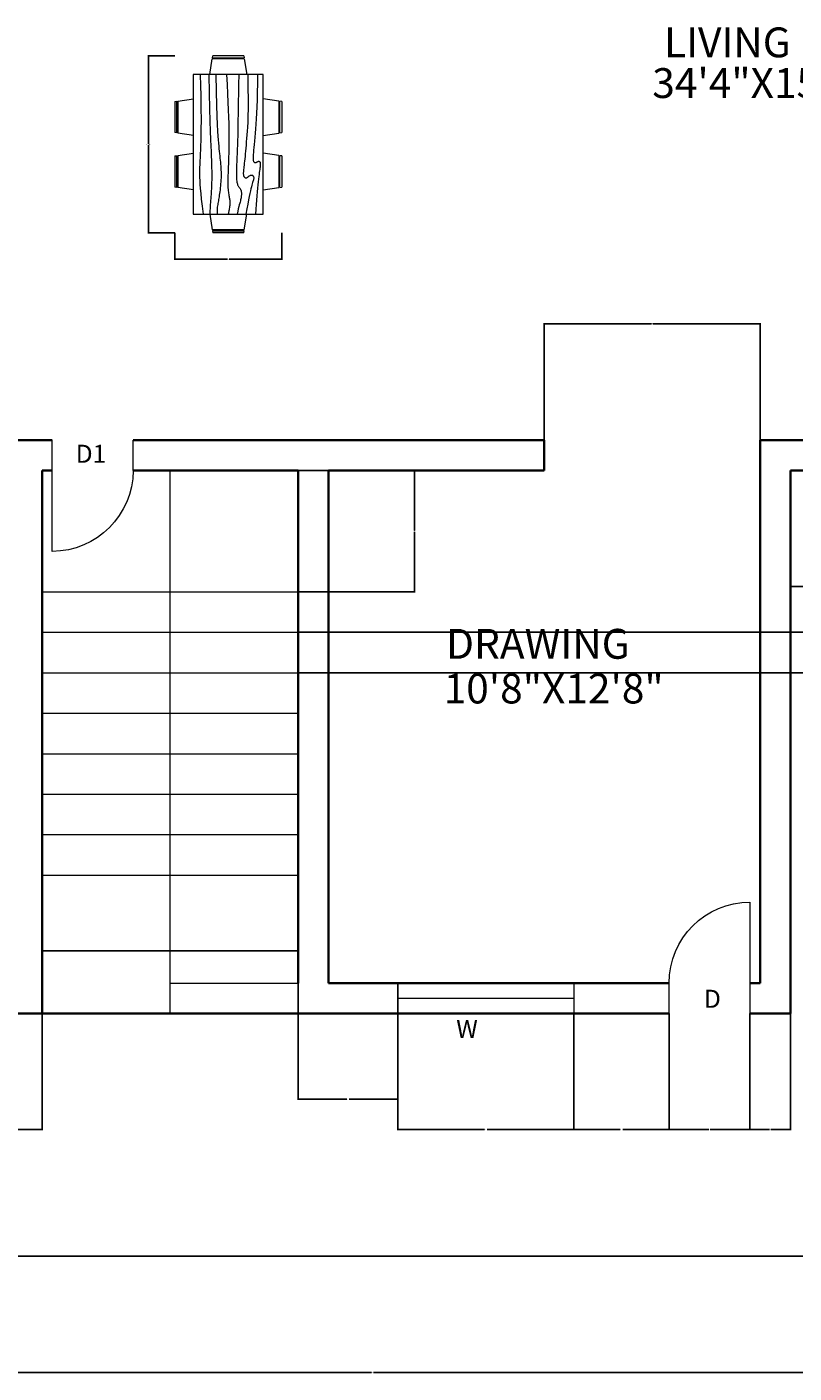
# Model space of a CAD drawing. Units: feet. Extents: x 1508 to 2265, y 1718 to 2421.
# Tile 2 of 4: x 1784 to 2012, y 1718 to 2117. Entities that reach past the tile are written whole.
import ezdxf

# ---------------------------------------------------------------- set-up
doc = ezdxf.new("R2010")
doc.units = ezdxf.units.FT
for name, color, linetype, lineweight in [('A-ANNO-DIMS', 2, 'Continuous', 18), ('A-ANNO-TEXT', 3, 'Continuous', 13), ('A-AREA-IDEN', 7, 'Continuous', 18), ('A-DOOR', 3, 'Continuous', 18), ('A-FLOR-STRS', 2, 'Continuous', 18), ('A-FURN', 8, 'Continuous', 18), ('A-GLAZ', 4, 'Continuous', 18), ('A-WALL', 7, 'Continuous', 35), ('C-PROP', 7, 'Continuous', 25)]:
    doc.layers.add(name, color=color, linetype=linetype, lineweight=lineweight)
doc.styles.get("Standard").update_dxf_attribs({"font": 'arial.ttf'})
doc.dimstyles.get("Standard").update_dxf_attribs({"dimtxt": 0.18, "dimasz": 0.18, "dimexe": 0.18, "dimexo": 0.0625, "dimgap": 0.09, "dimtad": 0, "dimtih": 1, "dimtoh": 1, "dimdec": 4, "dimzin": 0, "dimdsep": 46, "dimtxsty": 'Standard', "dimcen": 0.09, "dimadec": 0, "dimazin": 0, "dimtfac": 1, "dimtdec": 4, "dimtofl": 0, "dimtmove": 0, "dimatfit": 3, "dimfxl": 1, "dimtolj": 1, "dimtzin": 0, "dimarcsym": 0})

# ---------------------------------------------------------------- blocks, each defined once
blk = doc.blocks.new('Dining Set - 36 x 72 in.')
for p, q in [((-22.2343, 26.00059), (-23.4847, 17.99762)), ((-22.2304, 26), (-5.7608, 26)), ((-22, 27.5), (-22.1562, 26.50042)), ((-5.8416, 26.5), (-22.1534, 26.5)), ((-22, 27.5), (-6, 27.5)), ((-5.8437, 26.49966), (-6, 27.5)), ((-4.5152, 17.99762), (-5.7655, 25.99926)), ((5.7657, 26.00059), (4.5153, 17.99762)), ((5.7696, 26), (22.2392, 26)), ((6, 27.5), (5.8438, 26.50042)), ((22.1584, 26.5), (5.8466, 26.5)), ((6, 27.5), (22, 27.5)), ((22.1563, 26.49966), (22, 27.5)), ((23.4848, 17.99762), (22.2345, 25.99926)), ((36, 18), (-36, 18)), ((-36, 18), (-36, -18)), ((36, -18), (36, 18)), ((-45.5, 8), (-44.5004, 8.15617)), ((-45.5, 8), (-45.5, -8)), ((-44.5, -8.15843), (-44.5, 8.15338)), ((-44.0006, 8.23428), (-35.9976, 9.48474)), ((-44, 8.23041), (-44, -8.23915)), ((44.0006, 8.23428), (35.9976, 9.48474)), ((44, 8.23041), (44, -8.23915)), ((44.5, -8.15843), (44.5, 8.15338)), ((45.5, 8), (44.5005, 8.15617)), ((45.5, 8), (45.5, -8)), ((-44.4997, -8.15631), (-45.5, -8)), ((-35.9976, -9.48476), (-43.9993, -8.2345)), ((35.9976, -9.48476), (43.9993, -8.2345)), ((44.4997, -8.15631), (45.5, -8)), ((-36, -18), (36, -18)), ((-22.2343, -26.0006), (-23.4847, -17.99762)), ((-4.5152, -17.99762), (-5.7655, -25.99928)), ((5.7657, -26.0006), (4.5153, -17.99762)), ((23.4848, -17.99762), (22.2345, -25.99928)), ((-22.2304, -26), (-5.7608, -26)), ((-22, -27.5), (-22.1562, -26.50044)), ((-5.8416, -26.5), (-22.1534, -26.5)), ((-22, -27.5), (-6, -27.5)), ((-5.8437, -26.49967), (-6, -27.5)), ((5.7696, -26), (22.2392, -26)), ((6, -27.5), (5.8438, -26.50044)), ((22.1584, -26.5), (5.8466, -26.5)), ((6, -27.5), (22, -27.5)), ((22.1563, -26.49967), (22, -27.5))]:
    blk.add_line(p, q)
for points in [[(-36, 15), (-31.1772, 14.97754), (-26.8079, 14.91406), (-22.8538, 14.81543), (-19.276, 14.6875), (-16.0362, 14.53613), (-13.0957, 14.36718), (-10.4159, 14.18652), (-7.9583, 14), (-5.6904, 13.81315), (-3.6035, 13.63021), (-1.6954, 13.45508), (0.0365, 13.29166), (1.5945, 13.14388), (2.9811, 13.01562), (4.1988, 12.9108), (5.25, 12.83333), (6.1393, 12.78613), (6.8802, 12.76823), (7.4883, 12.77767), (7.9792, 12.8125), (8.3685, 12.87077), (8.6719, 12.95052), (8.9049, 13.0498), (9.0833, 13.16666), (9.2205, 13.29899), (9.3216, 13.44401), (9.3895, 13.59879), (9.4271, 13.76041), (9.4373, 13.92594), (9.4232, 14.09245), (9.3875, 14.257), (9.3333, 14.41666), (9.2638, 14.56917), (9.1836, 14.71484), (9.0975, 14.85465), (9.0104, 14.98958), (8.9272, 15.1206), (8.8529, 15.2487), (8.7922, 15.37483), (8.75, 15.5), (8.7305, 15.62467), (8.7344, 15.74739), (8.7617, 15.86621), (8.8125, 15.97916), (8.8867, 16.08431), (8.9844, 16.17968), (9.1055, 16.26334), (9.25, 16.33333), (9.4189, 16.38802), (9.6172, 16.42708), (9.8506, 16.45052), (10.125, 16.45833), (10.4463, 16.45052), (10.8203, 16.42708), (11.2529, 16.38802), (11.75, 16.33333), (12.3184, 16.26318), (12.9694, 16.17838), (13.7151, 16.07991), (14.5677, 15.96875), (15.5395, 15.84586), (16.6426, 15.71224), (17.8893, 15.56884), (19.2917, 15.41666), (20.859, 15.25667), (22.5879, 15.08984), (24.4721, 14.91715), (26.5052, 14.73958), (28.6809, 14.5581), (30.9929, 14.3737), (33.4347, 14.18733), (36, 14)], [(-36, 10), (-28.9766, 10.14274), (-23.1725, 10.20442), (-18.4241, 10.19775), (-14.5677, 10.13541), (-11.4399, 10.03011), (-8.877, 9.89453), (-6.7154, 9.74137), (-4.7917, 9.58333), (-2.9698, 9.43082), (-1.2246, 9.28515), (0.4415, 9.14534), (2.026, 9.01041), (3.5266, 8.87939), (4.9408, 8.7513), (6.266, 8.62516), (7.5, 8.5), (8.6411, 8.37549), (9.6914, 8.2539), (10.6538, 8.13818), (11.5312, 8.03125), (12.3267, 7.93603), (13.043, 7.85547), (13.6831, 7.79248), (14.25, 7.75), (14.7471, 7.7303), (15.1797, 7.73307), (15.5537, 7.75732), (15.875, 7.80208), (16.1494, 7.86637), (16.3828, 7.94922), (16.5811, 8.04964), (16.75, 8.16666), (16.8944, 8.29915), (17.0143, 8.44531), (17.1089, 8.60319), (17.1771, 8.77083), (17.218, 8.94629), (17.2305, 9.1276), (17.2137, 9.31282), (17.1667, 9.5), (17.0895, 9.6875), (16.987, 9.875), (16.8649, 10.0625), (16.7292, 10.25), (16.5856, 10.4375), (16.4401, 10.625), (16.2985, 10.8125), (16.1667, 11), (16.05, 11.18733), (15.9518, 11.3737), (15.8752, 11.5581), (15.8229, 11.73958), (15.798, 11.91715), (15.8034, 12.08984), (15.842, 12.25667), (15.9167, 12.41666), (16.0295, 12.56836), (16.1784, 12.70833), (16.3605, 12.83268), (16.5729, 12.9375), (16.8127, 13.01888), (17.0768, 13.07291), (17.3625, 13.0957), (17.6667, 13.08333), (17.9894, 13.03312), (18.3418, 12.94726), (18.7382, 12.82918), (19.1927, 12.68229), (19.7195, 12.51001), (20.3327, 12.31575), (21.0465, 12.10294), (21.875, 11.875), (22.8357, 11.63354), (23.959, 11.37304), (25.2786, 11.08618), (26.8282, 10.76562), (28.6414, 10.40405), (30.752, 9.99414), (33.1936, 9.52856), (36, 9)], [(-36, 5.5), (-30.7157, 5.3348), (-26.069, 5.20963), (-21.9946, 5.11767), (-18.4271, 5.05208), (-15.3009, 5.00602), (-12.5508, 4.97265), (-10.1112, 4.94515), (-7.9167, 4.91666), (-5.909, 4.88167), (-4.0586, 4.83984), (-2.3429, 4.79215), (-0.7396, 4.73958), (0.7739, 4.6831), (2.22, 4.6237), (3.6213, 4.56233), (5, 4.5), (6.373, 4.43782), (7.7344, 4.3776), (9.0723, 4.32129), (10.375, 4.27083), (11.6309, 4.22819), (12.8281, 4.19531), (13.9551, 4.17415), (15, 4.16666), (15.954, 4.17448), (16.819, 4.19791), (17.6001, 4.23698), (18.3021, 4.29166), (18.9299, 4.36198), (19.4883, 4.44791), (19.9823, 4.54948), (20.4167, 4.66666), (20.7969, 4.79899), (21.1302, 4.94401), (21.4245, 5.09879), (21.6875, 5.26041), (21.9271, 5.42594), (22.1511, 5.59245), (22.3672, 5.757), (22.5834, 5.91666), (22.8065, 6.06868), (23.0404, 6.21093), (23.2879, 6.34147), (23.5521, 6.45833), (23.8358, 6.55957), (24.142, 6.64323), (24.4735, 6.70735), (24.8334, 6.75), (25.2235, 6.76969), (25.642, 6.76692), (26.0858, 6.74267), (26.5521, 6.69791), (27.0379, 6.63362), (27.5404, 6.55078), (28.0565, 6.45036), (28.5834, 6.33333), (29.1242, 6.19987), (29.7071, 6.04687), (30.3661, 5.87044), (31.1354, 5.66666), (32.0493, 5.43164), (33.142, 5.16146), (34.4475, 4.85221), (36, 4.5)], [(-36, -1), (-30.7915, -0.6591), (-26.0195, -0.38216), (-21.6519, -0.16284), (-17.6563, 0.00521), (-14.0005, 0.12833), (-10.6523, 0.21289), (-7.5796, 0.26522), (-4.75, 0.29166), (-2.134, 0.29793), (0.2878, 0.28711), (2.5317, 0.26163), (4.6146, 0.22396), (6.5529, 0.17651), (8.3633, 0.12174), (10.0623, 0.06209), (11.6667, 0), (13.1899, -0.06201), (14.6341, -0.1211), (15.9982, -0.17432), (17.2813, -0.21875), (18.4823, -0.25147), (19.6003, -0.26953), (20.6343, -0.27002), (21.5834, -0.25), (22.4481, -0.20768), (23.2357, -0.14584), (23.9549, -0.06836), (24.6146, 0.02083), (25.2235, 0.11784), (25.7904, 0.21875), (26.3241, 0.31966), (26.8334, 0.41666), (27.3265, 0.50618), (27.8099, 0.58593), (28.2894, 0.65397), (28.7709, 0.70833), (29.2601, 0.74707), (29.763, 0.76823), (30.2855, 0.76985), (30.8334, 0.75), (31.4088, 0.70784), (31.9994, 0.64713), (32.589, 0.57275), (33.1615, 0.48958), (33.7008, 0.4025), (34.1908, 0.3164), (34.6153, 0.23616), (34.9584, 0.16666), (35.2099, 0.11165), (35.3848, 0.07031), (35.504, 0.04069), (35.5886, 0.02083), (35.6594, 0.00879), (35.7377, 0.0026), (35.8442, 0.00032), (36, 0)], [(-36, -6.5), (-27.1843, -6.31267), (-20.084, -6.1263), (-14.469, -5.9419), (-10.1094, -5.76042), (-6.7752, -5.58285), (-4.2363, -5.41016), (-2.2629, -5.24333), (-0.625, -5.08334), (0.8708, -4.93099), (2.2715, -4.78646), (3.5872, -4.64974), (4.8281, -4.52084), (6.0046, -4.39974), (7.127, -4.28646), (8.2053, -4.18099), (9.25, -4.08334), (10.2705, -3.99382), (11.2734, -3.91407), (12.2647, -3.84603), (13.25, -3.79167), (14.2354, -3.75293), (15.2266, -3.73177), (16.2295, -3.73015), (17.25, -3.75), (18.2912, -3.79248), (19.3451, -3.85547), (20.4009, -3.93604), (21.4479, -4.03125), (22.4754, -4.13819), (23.4727, -4.25391), (24.4289, -4.37549), (25.3334, -4.5), (26.1785, -4.62492), (26.9694, -4.74935), (27.7145, -4.87281), (28.4219, -4.99479), (29.1, -5.11483), (29.7572, -5.23242), (30.4016, -5.34709), (31.0417, -5.45834), (31.6837, -5.56437), (32.3262, -5.65821), (32.9658, -5.73153), (33.599, -5.77604), (34.2224, -5.78345), (34.8327, -5.74545), (35.4264, -5.65373), (36, -5.5)], [(-36, -10), (-26.4022, -9.81299), (-18.4675, -9.62891), (-11.9839, -9.45069), (-6.7396, -9.28125), (-2.5226, -9.12354), (0.8789, -8.98047), (3.6769, -8.85498), (6.0833, -8.75), (8.2767, -8.66765), (10.3021, -8.60677), (12.1712, -8.56543), (13.8958, -8.54167), (15.4876, -8.53353), (16.9583, -8.53907), (18.3197, -8.55632), (19.5834, -8.58334), (20.7616, -8.61841), (21.8685, -8.66081), (22.9188, -8.71004), (23.9271, -8.76563), (24.9081, -8.82707), (25.8763, -8.89388), (26.8465, -8.96558), (27.8334, -9.04167), (28.8474, -9.12118), (29.8828, -9.20117), (30.93, -9.27824), (31.9792, -9.34896), (33.0205, -9.40991), (34.0443, -9.45768), (35.0407, -9.48885), (36, -9.5)], [(-36, -14.5), (-30.0881, -14.33513), (-25.0332, -14.21224), (-20.7312, -14.12647), (-17.0781, -14.07292), (-13.97, -14.04671), (-11.3027, -14.04297), (-8.9724, -14.05681), (-6.875, -14.08334), (-4.9224, -14.11833), (-3.0905, -14.16016), (-1.3709, -14.20785), (0.2448, -14.26042), (1.7647, -14.3169), (3.1973, -14.3763), (4.5507, -14.43767), (5.8333, -14.5), (7.0554, -14.5621), (8.235, -14.62175), (9.3922, -14.67652), (10.5469, -14.72396), (11.7192, -14.76164), (12.929, -14.78711), (14.1965, -14.79794), (15.5417, -14.79167), (16.9933, -14.76424), (18.6152, -14.70508), (20.4804, -14.60197), (22.6615, -14.44271), (25.2312, -14.21509), (28.2624, -13.9069), (31.8277, -13.50594), (36, -13)]]:
    blk.add_lwpolyline(points)
blk = doc.blocks.new('DOOR-LEAF-24')
blk.add_line((0, 33), (0, 0))
blk.add_arc((0, 9), 24, 0, 90)
blk = doc.blocks.new('*D25')
at = {"layer": 'A-ANNO-DIMS', "color": 0, "lineweight": -2, "transparency": 16777216}
for p, q in [((1828.14, 2108.16), (1820.16, 2108.16)), ((1820.34, 2107.98), (1820.34, 2082.13)), ((1820.34, 2055.91), (1820.34, 2081.76)), ((1828.14, 2055.73), (1820.16, 2055.73))]:
    blk.add_line(p, q, dxfattribs=at)
at = {"layer": 'A-ANNO-DIMS', "color": 0, "transparency": 16777216}
for points in [[(1820.31, 2107.98), (1820.37, 2107.98), (1820.34, 2108.16)], [(1820.31, 2055.91), (1820.37, 2055.91), (1820.34, 2055.73)]]:
    blk.add_solid(points, dxfattribs=at)
at = {"layer": 'Defpoints', "color": 0, "transparency": 16777216}
for p in [(1828.2, 2108.16), (1820.34, 2055.73), (1828.2, 2055.73)]:
    blk.add_point(p, dxfattribs=at)
at = {"layer": 'A-ANNO-DIMS', "color": 0, "transparency": 16777216, "insert": (1820.34, 2081.95), "char_height": 0.18, "attachment_point": 5}
blk.add_mtext('\\A1;DINING SET 52', dxfattribs=at)
blk = doc.blocks.new('*D26')
at = {"layer": 'A-ANNO-DIMS', "color": 0, "lineweight": -2, "transparency": 16777216}
for p, q in [((1828.2, 2055.67), (1828.2, 2047.68)), ((1859.89, 2055.67), (1859.89, 2047.68)), ((1828.38, 2047.86), (1843.83, 2047.86)), ((1859.71, 2047.86), (1844.27, 2047.86))]:
    blk.add_line(p, q, dxfattribs=at)
at = {"layer": 'A-ANNO-DIMS', "color": 0, "transparency": 16777216}
for points in [[(1828.38, 2047.89), (1828.38, 2047.83), (1828.2, 2047.86)], [(1859.71, 2047.89), (1859.71, 2047.83), (1859.89, 2047.86)]]:
    blk.add_solid(points, dxfattribs=at)
at = {"layer": 'Defpoints', "color": 0, "transparency": 16777216}
for p in [(1828.2, 2055.73), (1859.89, 2055.73), (1859.89, 2047.86)]:
    blk.add_point(p, dxfattribs=at)
at = {"layer": 'A-ANNO-DIMS', "color": 0, "transparency": 16777216, "insert": (1844.05, 2047.86), "char_height": 0.18, "attachment_point": 5}
blk.add_mtext('\\A1;32', dxfattribs=at)
blk = doc.blocks.new('*D31')
at = {"layer": 'A-ANNO-DIMS', "color": 0, "lineweight": -2, "transparency": 16777216}
for p, q in [((1542.8, 1752.2), (1542.8, 1717.61)), ((2230.8, 1752.2), (2230.8, 1717.61)), ((1542.98, 1717.79), (1886.52, 1717.79)), ((2230.62, 1717.79), (1887.09, 1717.79))]:
    blk.add_line(p, q, dxfattribs=at)
at = {"layer": 'A-ANNO-DIMS', "color": 0, "transparency": 16777216}
for points in [[(1542.98, 1717.82), (1542.98, 1717.76), (1542.8, 1717.79)], [(2230.62, 1717.82), (2230.62, 1717.76), (2230.8, 1717.79)]]:
    blk.add_solid(points, dxfattribs=at)
at = {"layer": 'Defpoints', "color": 0, "transparency": 16777216}
for p in [(1542.8, 1752.26), (2230.8, 1752.26), (2230.8, 1717.79)]:
    blk.add_point(p, dxfattribs=at)
at = {"layer": 'A-ANNO-DIMS', "color": 0, "transparency": 16777216, "insert": (1886.8, 1717.79), "char_height": 0.18, "attachment_point": 5}
blk.add_mtext('\\A1;688', dxfattribs=at)
blk = doc.blocks.new('*D68')
at = {"layer": 'A-ANNO-DIMS', "color": 0, "lineweight": -2, "transparency": 16777216}
for p, q in [((1750.65, 1824.2), (1750.65, 1789.61)), ((1788.8, 1824.2), (1788.8, 1789.61)), ((1750.83, 1789.79), (1769.33, 1789.79)), ((1788.62, 1789.79), (1770.12, 1789.79))]:
    blk.add_line(p, q, dxfattribs=at)
at = {"layer": 'A-ANNO-DIMS', "color": 0, "transparency": 16777216}
for points in [[(1750.83, 1789.82), (1750.83, 1789.76), (1750.65, 1789.79)], [(1788.62, 1789.82), (1788.62, 1789.76), (1788.8, 1789.79)]]:
    blk.add_solid(points, dxfattribs=at)
at = {"layer": 'Defpoints', "color": 0, "transparency": 16777216}
for p in [(1750.65, 1824.26), (1788.8, 1824.26), (1750.65, 1789.79)]:
    blk.add_point(p, dxfattribs=at)
at = {"layer": 'A-ANNO-DIMS', "color": 0, "transparency": 16777216, "insert": (1769.73, 1789.79), "char_height": 0.18, "attachment_point": 5}
blk.add_mtext('\\A1;38.15', dxfattribs=at)
blk = doc.blocks.new('*D69')
at = {"layer": 'A-ANNO-DIMS', "color": 0, "lineweight": -2, "transparency": 16777216}
for p, q in [((1788.8, 1877.2), (1788.8, 1842.61)), ((1864.8, 1877.2), (1864.8, 1842.61)), ((1788.98, 1842.79), (1826.59, 1842.79)), ((1864.62, 1842.79), (1827.02, 1842.79))]:
    blk.add_line(p, q, dxfattribs=at)
at = {"layer": 'A-ANNO-DIMS', "color": 0, "transparency": 16777216}
for points in [[(1788.98, 1842.82), (1788.98, 1842.76), (1788.8, 1842.79)], [(1864.62, 1842.82), (1864.62, 1842.76), (1864.8, 1842.79)]]:
    blk.add_solid(points, dxfattribs=at)
at = {"layer": 'Defpoints', "color": 0, "transparency": 16777216}
for p in [(1788.8, 1877.26), (1864.8, 1877.26), (1788.8, 1842.79)]:
    blk.add_point(p, dxfattribs=at)
at = {"layer": 'A-ANNO-DIMS', "color": 0, "transparency": 16777216, "insert": (1826.8, 1842.79), "char_height": 0.18, "attachment_point": 5}
blk.add_mtext('\\A1;76', dxfattribs=at)
blk = doc.blocks.new('*D70')
at = {"layer": 'A-ANNO-DIMS', "color": 0, "lineweight": -2, "transparency": 16777216}
for p, q in [((1864.8, 1833.2), (1864.8, 1798.61)), ((1894.31, 1833.2), (1894.31, 1798.61)), ((1864.98, 1798.79), (1879.23, 1798.79)), ((1894.13, 1798.79), (1879.88, 1798.79))]:
    blk.add_line(p, q, dxfattribs=at)
at = {"layer": 'A-ANNO-DIMS', "color": 0, "transparency": 16777216}
for points in [[(1864.98, 1798.82), (1864.98, 1798.76), (1864.8, 1798.79)], [(1894.13, 1798.82), (1894.13, 1798.76), (1894.31, 1798.79)]]:
    blk.add_solid(points, dxfattribs=at)
at = {"layer": 'Defpoints', "color": 0, "transparency": 16777216}
for p in [(1864.8, 1833.26), (1894.31, 1833.26), (1864.8, 1798.79)]:
    blk.add_point(p, dxfattribs=at)
at = {"layer": 'A-ANNO-DIMS', "color": 0, "transparency": 16777216, "insert": (1879.56, 1798.79), "char_height": 0.18, "attachment_point": 5}
blk.add_mtext('\\A1;29.5', dxfattribs=at)
blk = doc.blocks.new('*D71')
at = {"layer": 'A-ANNO-DIMS', "color": 0, "lineweight": -2, "transparency": 16777216}
for p, q in [((1894.31, 1824.2), (1894.31, 1789.61)), ((1946.55, 1824.2), (1946.55, 1789.61)), ((1894.49, 1789.79), (1920.03, 1789.79)), ((1946.37, 1789.79), (1920.82, 1789.79))]:
    blk.add_line(p, q, dxfattribs=at)
at = {"layer": 'A-ANNO-DIMS', "color": 0, "transparency": 16777216}
for points in [[(1894.49, 1789.82), (1894.49, 1789.76), (1894.31, 1789.79)], [(1946.37, 1789.82), (1946.37, 1789.76), (1946.55, 1789.79)]]:
    blk.add_solid(points, dxfattribs=at)
at = {"layer": 'Defpoints', "color": 0, "transparency": 16777216}
for p in [(1894.31, 1824.26), (1946.55, 1824.26), (1894.31, 1789.79)]:
    blk.add_point(p, dxfattribs=at)
at = {"layer": 'A-ANNO-DIMS', "color": 0, "transparency": 16777216, "insert": (1920.43, 1789.79), "char_height": 0.18, "attachment_point": 5}
blk.add_mtext('\\A1;52.25', dxfattribs=at)
blk = doc.blocks.new('*D72')
at = {"layer": 'A-ANNO-DIMS', "color": 0, "lineweight": -2, "transparency": 16777216}
for p, q in [((1946.55, 1824.2), (1946.55, 1789.61)), ((1974.8, 1824.2), (1974.8, 1789.61)), ((1946.73, 1789.79), (1960.28, 1789.79)), ((1974.62, 1789.79), (1961.07, 1789.79))]:
    blk.add_line(p, q, dxfattribs=at)
at = {"layer": 'A-ANNO-DIMS', "color": 0, "transparency": 16777216}
for points in [[(1946.73, 1789.82), (1946.73, 1789.76), (1946.55, 1789.79)], [(1974.62, 1789.82), (1974.62, 1789.76), (1974.8, 1789.79)]]:
    blk.add_solid(points, dxfattribs=at)
at = {"layer": 'Defpoints', "color": 0, "transparency": 16777216}
for p in [(1946.55, 1824.26), (1974.8, 1824.26), (1946.55, 1789.79)]:
    blk.add_point(p, dxfattribs=at)
at = {"layer": 'A-ANNO-DIMS', "color": 0, "transparency": 16777216, "insert": (1960.68, 1789.79), "char_height": 0.18, "attachment_point": 5}
blk.add_mtext('\\A1;28.25', dxfattribs=at)
blk = doc.blocks.new('*D73')
at = {"layer": 'A-ANNO-DIMS', "color": 0, "lineweight": -2, "transparency": 16777216}
for p, q in [((1974.8, 1824.2), (1974.8, 1789.61)), ((1998.8, 1824.2), (1998.8, 1789.61)), ((1974.98, 1789.79), (1986.58, 1789.79)), ((1998.62, 1789.79), (1987.02, 1789.79))]:
    blk.add_line(p, q, dxfattribs=at)
at = {"layer": 'A-ANNO-DIMS', "color": 0, "transparency": 16777216}
for points in [[(1974.98, 1789.82), (1974.98, 1789.76), (1974.8, 1789.79)], [(1998.62, 1789.82), (1998.62, 1789.76), (1998.8, 1789.79)]]:
    blk.add_solid(points, dxfattribs=at)
at = {"layer": 'Defpoints', "color": 0, "transparency": 16777216}
for p in [(1974.8, 1824.26), (1998.8, 1824.26), (1974.8, 1789.79)]:
    blk.add_point(p, dxfattribs=at)
at = {"layer": 'A-ANNO-DIMS', "color": 0, "transparency": 16777216, "insert": (1986.8, 1789.79), "char_height": 0.18, "attachment_point": 5}
blk.add_mtext('\\A1;24', dxfattribs=at)
blk = doc.blocks.new('*D74')
at = {"layer": 'A-ANNO-DIMS', "color": 0, "lineweight": -2, "transparency": 16777216}
for p, q in [((1998.8, 1824.2), (1998.8, 1789.61)), ((2010.8, 1824.2), (2010.8, 1789.61)), ((1998.98, 1789.79), (2004.6, 1789.79)), ((2010.62, 1789.79), (2005.01, 1789.79))]:
    blk.add_line(p, q, dxfattribs=at)
at = {"layer": 'A-ANNO-DIMS', "color": 0, "transparency": 16777216}
for points in [[(1998.98, 1789.82), (1998.98, 1789.76), (1998.8, 1789.79)], [(2010.62, 1789.82), (2010.62, 1789.76), (2010.8, 1789.79)]]:
    blk.add_solid(points, dxfattribs=at)
at = {"layer": 'Defpoints', "color": 0, "transparency": 16777216}
for p in [(1998.8, 1824.26), (2010.8, 1824.26), (1998.8, 1789.79)]:
    blk.add_point(p, dxfattribs=at)
at = {"layer": 'A-ANNO-DIMS', "color": 0, "transparency": 16777216, "insert": (2004.8, 1789.79), "char_height": 0.18, "attachment_point": 5}
blk.add_mtext('\\A1;12', dxfattribs=at)
blk = doc.blocks.new('*D75')
at = {"layer": 'A-ANNO-DIMS', "color": 0, "lineweight": -2, "transparency": 16777216}
for p, q in [((2010.8, 1985.2), (2010.8, 1950.61)), ((2062.3, 1985.2), (2062.3, 1950.61)), ((2010.98, 1950.79), (2036.23, 1950.79)), ((2062.12, 1950.79), (2036.88, 1950.79))]:
    blk.add_line(p, q, dxfattribs=at)
at = {"layer": 'A-ANNO-DIMS', "color": 0, "transparency": 16777216}
for points in [[(2010.98, 1950.82), (2010.98, 1950.76), (2010.8, 1950.79)], [(2062.12, 1950.82), (2062.12, 1950.76), (2062.3, 1950.79)]]:
    blk.add_solid(points, dxfattribs=at)
at = {"layer": 'Defpoints', "color": 0, "transparency": 16777216}
for p in [(2010.8, 1985.26), (2062.3, 1985.26), (2010.8, 1950.79)]:
    blk.add_point(p, dxfattribs=at)
at = {"layer": 'A-ANNO-DIMS', "color": 0, "transparency": 16777216, "insert": (2036.55, 1950.79), "char_height": 0.18, "attachment_point": 5}
blk.add_mtext('\\A1;51.5', dxfattribs=at)
blk = doc.blocks.new('*D79')
at = {"layer": 'A-ANNO-DIMS', "color": 0, "lineweight": -2, "transparency": 16777216}
for p, q in [((1864.87, 1937.26), (2265.46, 1937.26)), ((2265.28, 1937.08), (2265.28, 1931.44)), ((2265.28, 1925.44), (2265.28, 1931.08)), ((1864.87, 1925.26), (2265.46, 1925.26))]:
    blk.add_line(p, q, dxfattribs=at)
at = {"layer": 'A-ANNO-DIMS', "color": 0, "transparency": 16777216}
for points in [[(2265.25, 1937.08), (2265.31, 1937.08), (2265.28, 1937.26)], [(2265.25, 1925.44), (2265.31, 1925.44), (2265.28, 1925.26)]]:
    blk.add_solid(points, dxfattribs=at)
at = {"layer": 'Defpoints', "color": 0, "transparency": 16777216}
for p in [(1864.8, 1937.26), (1864.8, 1925.26), (2265.28, 1925.26)]:
    blk.add_point(p, dxfattribs=at)
at = {"layer": 'A-ANNO-DIMS', "color": 0, "transparency": 16777216, "insert": (2265.28, 1931.26), "char_height": 0.18, "attachment_point": 5}
blk.add_mtext('\\A1;12', dxfattribs=at)
blk = doc.blocks.new('*D83')
at = {"layer": 'A-ANNO-DIMS', "color": 0, "lineweight": -2, "transparency": 16777216}
for p, q in [((1937.8, 1994.32), (1937.8, 2028.92)), ((1937.98, 2028.74), (1969.59, 2028.74)), ((2001.62, 2028.74), (1970.02, 2028.74)), ((2001.8, 1994.32), (2001.8, 2028.92))]:
    blk.add_line(p, q, dxfattribs=at)
at = {"layer": 'A-ANNO-DIMS', "color": 0, "transparency": 16777216}
for points in [[(1937.98, 2028.77), (1937.98, 2028.71), (1937.8, 2028.74)], [(2001.62, 2028.77), (2001.62, 2028.71), (2001.8, 2028.74)]]:
    blk.add_solid(points, dxfattribs=at)
at = {"layer": 'Defpoints', "color": 0, "transparency": 16777216}
for p in [(2001.8, 2028.74), (1937.8, 1994.26), (2001.8, 1994.26)]:
    blk.add_point(p, dxfattribs=at)
at = {"layer": 'A-ANNO-DIMS', "color": 0, "transparency": 16777216, "insert": (1969.8, 2028.74), "char_height": 0.18, "attachment_point": 5}
blk.add_mtext('\\A1;64', dxfattribs=at)
blk = doc.blocks.new('*D84')
at = {"layer": 'A-ANNO-DIMS', "color": 0, "lineweight": -2, "transparency": 16777216}
for p, q in [((1864.87, 1985.26), (1899.46, 1985.26)), ((1899.28, 1985.08), (1899.28, 1967.44)), ((1899.28, 1949.44), (1899.28, 1967.08)), ((1864.87, 1949.26), (1899.46, 1949.26))]:
    blk.add_line(p, q, dxfattribs=at)
at = {"layer": 'A-ANNO-DIMS', "color": 0, "transparency": 16777216}
for points in [[(1899.25, 1985.08), (1899.31, 1985.08), (1899.28, 1985.26)], [(1899.25, 1949.44), (1899.31, 1949.44), (1899.28, 1949.26)]]:
    blk.add_solid(points, dxfattribs=at)
at = {"layer": 'Defpoints', "color": 0, "transparency": 16777216}
for p in [(1864.8, 1985.26), (1864.8, 1949.26), (1899.28, 1949.26)]:
    blk.add_point(p, dxfattribs=at)
at = {"layer": 'A-ANNO-DIMS', "color": 0, "transparency": 16777216, "insert": (1899.28, 1967.26), "char_height": 0.18, "attachment_point": 5}
blk.add_mtext('\\A1;36', dxfattribs=at)

msp = doc.modelspace()

# ---------------------------------------------------------------- linework, layer by layer
at = {"layer": 'A-DOOR'}
for p, q in [((1815.8049, 1985.2608), (1815.8049, 1994.2608)), ((1974.8049, 1824.2608), (1974.8049, 1833.2608))]:
    msp.add_line(p, q, dxfattribs=at)
at = {"layer": 'A-FLOR-STRS'}
for p, q in [((1826.8049, 1824.2608), (1826.8049, 1985.2608)), ((1788.8049, 1949.2608), (1864.8049, 1949.2608)), ((1788.8049, 1937.2608), (1864.8049, 1937.2608)), ((1788.8049, 1925.2608), (1864.8049, 1925.2608)), ((1788.8049, 1913.2608), (1864.8049, 1913.2608)), ((1788.8049, 1901.2608), (1864.8049, 1901.2608)), ((1788.8049, 1889.2608), (1864.8049, 1889.2608)), ((1788.8049, 1877.2608), (1864.8049, 1877.2608)), ((1788.8049, 1865.2608), (1864.8049, 1865.2608)), ((1826.8049, 1833.2608), (1864.8049, 1833.2608))]:
    msp.add_line(p, q, dxfattribs=at)
at = {"layer": 'A-GLAZ'}
for p, q in [((1894.3054, 1833.2608), (1894.3054, 1824.2608)), ((1946.5529, 1833.2608), (1946.5529, 1824.2608)), ((1894.3054, 1828.7608), (1946.5529, 1828.7608))]:
    msp.add_line(p, q, dxfattribs=at)
at = {"layer": 'A-WALL'}
for p, q in [((1776.8049, 1994.2608), (1791.8049, 1994.2608)), ((1815.8049, 1994.2608), (1937.8049, 1994.2608)), ((1937.8049, 1985.2608), (1937.8049, 1994.2608)), ((2001.8049, 1833.2608), (2001.8049, 1994.2608)), ((2001.8049, 1994.2608), (2062.3049, 1994.2608)), ((1788.8049, 1824.2608), (1788.8049, 1985.2608)), ((1788.8049, 1985.2608), (1791.8049, 1985.2608)), ((1788.8049, 1985.2608), (1791.8049, 1985.2608)), ((1815.8049, 1985.2608), (1864.8049, 1985.2608)), ((1815.8049, 1985.2608), (1864.8049, 1985.2608)), ((1864.8049, 1985.2608), (1864.8049, 1833.2608)), ((1873.8049, 1985.2608), (1873.8049, 1833.2608)), ((1937.8049, 1985.2608), (1873.8049, 1985.2608)), ((1873.8049, 1985.2608), (1937.8049, 1985.2608)), ((2010.8049, 1824.2608), (2010.8049, 1985.2608)), ((2010.8049, 1985.2608), (2062.3049, 1985.2608)), ((1873.8049, 1833.2608), (1974.8049, 1833.2608)), ((1998.8049, 1833.2608), (2001.8049, 1833.2608)), ((1611.8049, 1824.2608), (1974.8049, 1824.2608)), ((1788.8049, 1824.2608), (1974.8049, 1824.2608)), ((1873.8049, 1824.2608), (1974.8049, 1824.2608)), ((1998.8049, 1824.2608), (2010.8049, 1824.2608)), ((1998.8049, 1824.2608), (2010.8049, 1824.2608)), ((1998.8049, 1824.2608), (2010.8049, 1824.2608))]:
    msp.add_line(p, q, dxfattribs=at)
at = {"layer": 'C-PROP'}
msp.add_line((1611.8049, 1752.2608), (2230.8049, 1752.2608), dxfattribs=at)

# ---------------------------------------------------------------- block references
at = {"layer": 'A-DOOR', "extrusion": (0, 0, -1), "zscale": -1, "rotation": 180}
msp.add_blockref('DOOR-LEAF-24', (-1791.805, 1994.2605), dxfattribs=at)
at = {"layer": 'A-DOOR', "extrusion": (0, 0, -1), "zscale": -1}
msp.add_blockref('DOOR-LEAF-24', (-1998.8048, 1824.261), dxfattribs=at)
at = {"layer": 'A-FURN', "xscale": 0.576213156998799, "yscale": 0.576213156998799, "zscale": 0.576213156998799, "rotation": 270}
msp.add_blockref('Dining Set - 36 x 72 in.', (1844.0487, 2081.9466), dxfattribs=at)

# ---------------------------------------------------------------- texts
at = {"layer": 'A-ANNO-TEXT'}
for s, height, p in [('D1', 5.34528, (1798.7858, 1987.5152)), ('D', 5.3453, (1985.1672, 1825.9111)), ('W', 5.3453, (1911.6674, 1816.9735))]:
    msp.add_text(s, height=height, dxfattribs=at).set_placement(p)
at = {"layer": 'A-AREA-IDEN'}
for s, height, p in [('LIVING', 8.85057, (1973.3039, 2107.7459)), ('34\'4"X15\'', 8.85057, (1969.8225, 2095.6807)), ('DRAWING', 8.85057, (1908.6474, 1929.4079)), ('10\'8"X12\'8"', 8.850571, (1907.9297, 1916.1606))]:
    msp.add_text(s, height=height, dxfattribs=at).set_placement(p)

# ---------------------------------------------------------------- dimensions: what is measured, and where the dimension line sits
at = {"layer": 'A-ANNO-DIMS'}
dim = msp.add_linear_dim(base=(1820.3375, 2055.7289), p1=(1828.2029, 2108.1643), p2=(1828.2029, 2055.7289), angle=270, text='DINING SET <>', dimstyle='Standard', override={"dimdec": 0, "dimlfac": 1, "dimrnd": 0, "dimzin": 0, "dimdsep": 46, "dimlunit": 2}, dxfattribs=at)
dim.commit()
dim.dimension.update_dxf_attribs({"geometry": '*D25', "text_midpoint": (1820.3375, 2081.9466)})
for base, p1, p2, picture, middle in [((1859.8946, 2047.8636), (1828.2029, 2055.7289), (1859.8946, 2055.7289), '*D26', (1844.0487, 2047.8636)), ((2001.8049, 2028.7358), (1937.8049, 1994.2608), (2001.8049, 1994.2608), '*D83', (1969.8049, 2028.7358)), ((2230.8049, 1717.7858), (1542.8049, 1752.2608), (2230.8049, 1752.2608), '*D31', (1886.8049, 1717.7858))]:
    dim = msp.add_linear_dim(base=base, p1=p1, p2=p2, dimstyle='Standard', override={"dimdec": 0, "dimlfac": 1, "dimrnd": 0, "dimzin": 0, "dimdsep": 46, "dimlunit": 2}, dxfattribs=at)
    dim.commit()
    dim.dimension.update_dxf_attribs({"geometry": picture, "text_midpoint": middle})
for base, p1, p2, angle, override, picture, middle in [((1899.2799, 1949.2608), (1864.8049, 1985.2608), (1864.8049, 1949.2608), 270, {"dimdec": 0, "dimlfac": 1, "dimrnd": 0, "dimzin": 0, "dimdsep": 46, "dimlunit": 2}, '*D84', (1899.2799, 1967.2608)), ((2010.8049, 1950.7858), (2062.3049, 1985.2608), (2010.8049, 1985.2608), 180, {"dimdec": 1, "dimlfac": 1, "dimrnd": 0, "dimzin": 0, "dimdsep": 46, "dimlunit": 2}, '*D75', (2036.5549, 1950.7858)), ((2265.2799, 1925.2608), (1864.8049, 1937.2608), (1864.8049, 1925.2608), 90, {"dimdec": 0, "dimlfac": 1, "dimrnd": 0, "dimzin": 0, "dimdsep": 46, "dimlunit": 2}, '*D79', (2265.2799, 1931.2608)), ((1788.8049, 1842.7858), (1864.8049, 1877.2608), (1788.8049, 1877.2608), 180, {"dimdec": 0, "dimlfac": 1, "dimrnd": 0, "dimzin": 0, "dimdsep": 46, "dimlunit": 2}, '*D69', (1826.8049, 1842.7858)), ((1864.8049, 1798.7858), (1894.3054, 1833.2608), (1864.8049, 1833.2608), 180, {"dimdec": 1, "dimlfac": 1, "dimrnd": 0, "dimzin": 0, "dimdsep": 46, "dimlunit": 2}, '*D70', (1879.5551, 1798.7858)), ((1750.6528, 1789.7858), (1788.8049, 1824.2608), (1750.6528, 1824.2608), 180, {"dimdec": 2, "dimlfac": 1, "dimrnd": 0, "dimzin": 0, "dimdsep": 46, "dimlunit": 2}, '*D68', (1769.7289, 1789.7858)), ((1894.3054, 1789.7858), (1946.5529, 1824.2608), (1894.3054, 1824.2608), 180, {"dimdec": 2, "dimlfac": 1, "dimrnd": 0, "dimzin": 0, "dimdsep": 46, "dimlunit": 2}, '*D71', (1920.4292, 1789.7858)), ((1946.5529, 1789.7858), (1974.8049, 1824.2608), (1946.5529, 1824.2608), 180, {"dimdec": 2, "dimlfac": 1, "dimrnd": 0, "dimzin": 0, "dimdsep": 46, "dimlunit": 2}, '*D72', (1960.6789, 1789.7858)), ((1974.8049, 1789.7858), (1998.8049, 1824.2608), (1974.8049, 1824.2608), 180, {"dimdec": 0, "dimlfac": 1, "dimrnd": 0, "dimzin": 0, "dimdsep": 46, "dimlunit": 2}, '*D73', (1986.8049, 1789.7858)), ((1998.8049, 1789.7858), (2010.8049, 1824.2608), (1998.8049, 1824.2608), 180, {"dimdec": 0, "dimlfac": 1, "dimrnd": 0, "dimzin": 0, "dimdsep": 46, "dimlunit": 2}, '*D74', (2004.8049, 1789.7858))]:
    dim = msp.add_linear_dim(base=base, p1=p1, p2=p2, angle=angle, dimstyle='Standard', override=override, dxfattribs=at)
    dim.commit()
    dim.dimension.update_dxf_attribs({"geometry": picture, "text_midpoint": middle})

doc.saveas('drawing.dxf')
